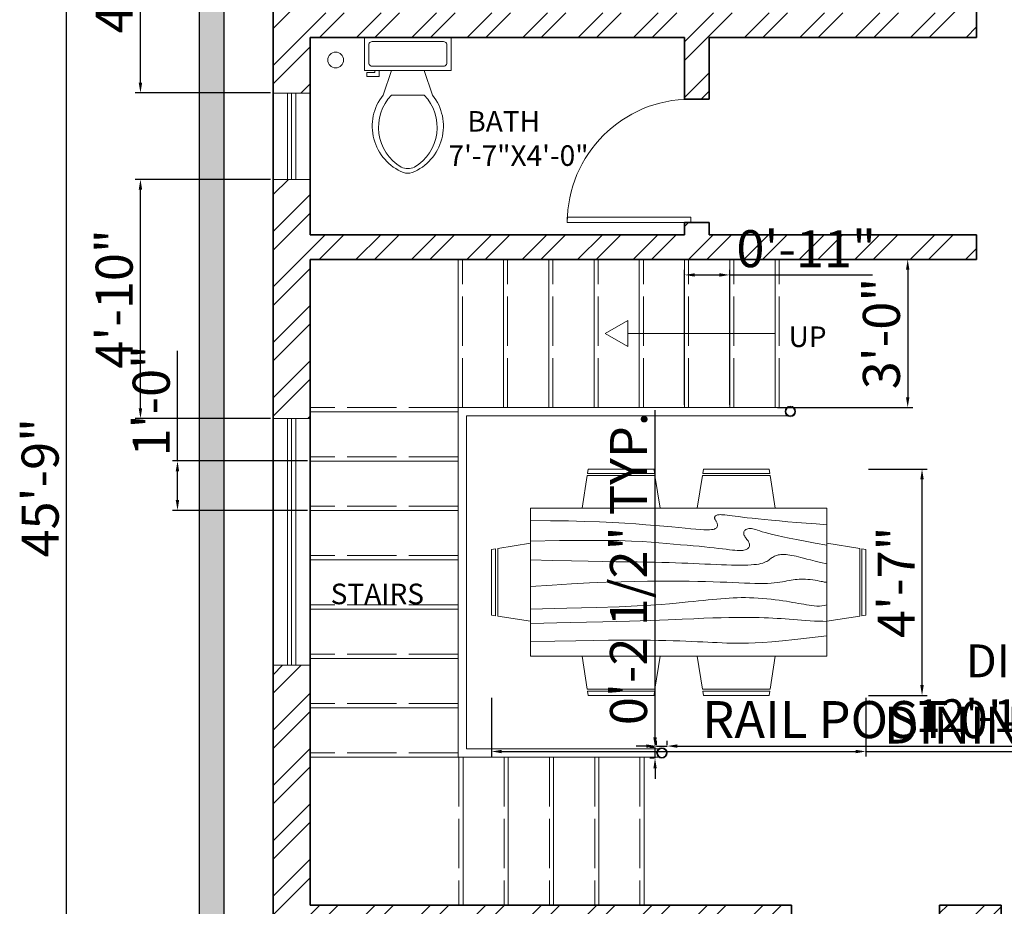
# Model space of a CAD drawing. Units: inches. Extents: x 418 to 1041, y 2094 to 2761.
# Tile 2 of 5: x 484 to 723, y 2308 to 2523. Entities that reach past the tile are written whole.
import ezdxf

# ---------------------------------------------------------------- set-up
doc = ezdxf.new("R2010")
doc.units = ezdxf.units.IN
doc.linetypes.add('ACAD_ISO02W100', pattern=[15, 12, -3])
for name, color, linetype, lineweight in [('A-ANNO-DIMS', 2, 'Continuous', 18), ('A-ANNO-SYMB', 7, 'Continuous', 18), ('A-ANNO-TEXT', 7, 'Continuous', 18), ('A-AREA-IDEN', 7, 'Continuous', 18), ('A-DOOR', 4, 'Continuous', 18), ('A-FLOR-FIXT', 9, 'Continuous', 18), ('A-FLOR-STRS', 7, 'Continuous', 18), ('A-FLOR-STRS-HIDN', 8, 'ACAD_ISO02W100', 13), ('A-FURN', 8, 'Continuous', 18), ('A-GLAZ', 244, 'Continuous', 18), ('A-WALL', 7, 'Continuous', 35), ('A-WALL-PATT', 252, 'Continuous', 13), ('L-WALL', 7, 'Continuous', 25), ('L-WALL-PATT', 252, 'Continuous', 13)]:
    doc.layers.add(name, color=color, linetype=linetype, lineweight=lineweight)
doc.styles.get("Standard").update_dxf_attribs({"font": 'arial.ttf'})
doc.dimstyles.new('ISO-25', dxfattribs={"dimtxt": 9, "dimasz": 2.5, "dimexe": 1.25, "dimexo": 0.625, "dimtad": 1, "dimlunit": 3, "dimtxsty": 'Standard', "dimcen": 2.5, "dimadec": 0, "dimazin": 0, "dimtfac": 1, "dimtmove": 0, "dimatfit": 3, "dimfxl": 1, "dimarcsym": 0})

# ---------------------------------------------------------------- blocks, each defined once
blk = doc.blocks.new('*U6')
for p, q in [((-40, 0), (-40, 6)), ((0, 0), (0, 6))]:
    blk.add_line(p, q)
blk.add_lwpolyline([(0, 0), (0, -40), (-1.75, -40), (-1.75, 0)], close=True)
blk.add_arc((0, 0), 40, 180, 270)
blk = doc.blocks.new('*U10')
for p, q in [((9.5, -6), (9.5, -2)), ((-10, -8.5), (-8, -8.5)), ((-10, -9.5), (-10, -8.5)), ((-7, -9.5), (-10, -9.5)), ((-8, -8.5), (-8, -8)), ((-7, -8), (-7, -9.5)), ((-4, -8), (-6, -14)), ((4, -8), (6, -14)), ((4, -14), (-4, -14))]:
    blk.add_line(p, q)
blk.add_lwpolyline([(10.5, -8), (10.5, 0), (-10.5, 0), (-10.5, -8)], close=True)
for points in [[(-9.5, -2), (-9.5, -6)], [(8.5, -1), (-8.5, -1)], [(-8.5, -7), (8.5, -7)]]:
    blk.add_lwpolyline(points)
for centre, radius, start, end in [((-8.62, -1.88), 0.884, 81.8699, 188.1301), ((8.62, -1.88), 0.884, 351.8699, 98.1301), ((-8.62, -6.12), 0.884, 171.8699, 278.1301), ((8.62, -6.12), 0.884, 261.8699, 8.1301), ((3.52, -21.58), 12.17, 141.4691, 247.9714), ((4.2, -21.82), 11.33, 136.3677, 238.9468), ((-3.52, -21.58), 12.17, 292.0284, 38.5307), ((-4.2, -21.82), 11.33, 301.053, 43.6321), ((0, -27.88), 4, 245.7318, 294.2682), ((0, -29), 4, 254.8605, 285.1395)]:
    blk.add_arc(centre, radius, start, end)
blk = doc.blocks.new('Dining Set - 36 x 72 in.')
for p, q in [((-22, 27.5), (-22.1562, 26.50042)), ((-5.8416, 26.5), (-22.1534, 26.5)), ((-22, 27.5), (-6, 27.5)), ((-5.8437, 26.49966), (-6, 27.5)), ((6, 27.5), (5.8438, 26.50042)), ((22.1584, 26.5), (5.8466, 26.5)), ((6, 27.5), (22, 27.5)), ((22.1563, 26.49966), (22, 27.5)), ((-22.2343, 26.00059), (-23.4847, 17.99762)), ((-22.2304, 26), (-5.7608, 26)), ((-4.5152, 17.99762), (-5.7655, 25.99926)), ((5.7657, 26.00059), (4.5153, 17.99762)), ((5.7696, 26), (22.2392, 26)), ((23.4848, 17.99762), (22.2345, 25.99926)), ((36, 18), (-36, 18)), ((-36, 18), (-36, -18)), ((36, -18), (36, 18)), ((-45.5, 8), (-44.5004, 8.15617)), ((-45.5, 8), (-45.5, -8)), ((-44.5, -8.15843), (-44.5, 8.15338)), ((-44.0006, 8.23428), (-35.9976, 9.48474)), ((-44, 8.23041), (-44, -8.23915)), ((44.0006, 8.23428), (35.9976, 9.48474)), ((44, 8.23041), (44, -8.23915)), ((44.5, -8.15843), (44.5, 8.15338)), ((45.5, 8), (44.5005, 8.15617)), ((45.5, 8), (45.5, -8)), ((-44.4997, -8.15631), (-45.5, -8)), ((-35.9976, -9.48476), (-43.9993, -8.2345)), ((35.9976, -9.48476), (43.9993, -8.2345)), ((44.4997, -8.15631), (45.5, -8)), ((-36, -18), (36, -18)), ((-22.2343, -26.0006), (-23.4847, -17.99762)), ((-4.5152, -17.99762), (-5.7655, -25.99928)), ((5.7657, -26.0006), (4.5153, -17.99762)), ((23.4848, -17.99762), (22.2345, -25.99928)), ((-22.2304, -26), (-5.7608, -26)), ((5.7696, -26), (22.2392, -26)), ((-22, -27.5), (-22.1562, -26.50044)), ((-5.8416, -26.5), (-22.1534, -26.5)), ((-22, -27.5), (-6, -27.5)), ((-5.8437, -26.49967), (-6, -27.5)), ((6, -27.5), (5.8438, -26.50044)), ((22.1584, -26.5), (5.8466, -26.5)), ((6, -27.5), (22, -27.5)), ((22.1563, -26.49967), (22, -27.5))]:
    blk.add_line(p, q)
for points in [[(-36, 15), (-31.1772, 14.97754), (-26.8079, 14.91406), (-22.8538, 14.81543), (-19.276, 14.6875), (-16.0362, 14.53613), (-13.0957, 14.36718), (-10.4159, 14.18652), (-7.9583, 14), (-5.6904, 13.81315), (-3.6035, 13.63021), (-1.6954, 13.45508), (0.0365, 13.29166), (1.5945, 13.14388), (2.9811, 13.01562), (4.1988, 12.9108), (5.25, 12.83333), (6.1393, 12.78613), (6.8802, 12.76823), (7.4883, 12.77767), (7.9792, 12.8125), (8.3685, 12.87077), (8.6719, 12.95052), (8.9049, 13.0498), (9.0833, 13.16666), (9.2205, 13.29899), (9.3216, 13.44401), (9.3895, 13.59879), (9.4271, 13.76041), (9.4373, 13.92594), (9.4232, 14.09245), (9.3875, 14.257), (9.3333, 14.41666), (9.2638, 14.56917), (9.1836, 14.71484), (9.0975, 14.85465), (9.0104, 14.98958), (8.9272, 15.1206), (8.8529, 15.2487), (8.7922, 15.37483), (8.75, 15.5), (8.7305, 15.62467), (8.7344, 15.74739), (8.7617, 15.86621), (8.8125, 15.97916), (8.8867, 16.08431), (8.9844, 16.17968), (9.1055, 16.26334), (9.25, 16.33333), (9.4189, 16.38802), (9.6172, 16.42708), (9.8506, 16.45052), (10.125, 16.45833), (10.4463, 16.45052), (10.8203, 16.42708), (11.2529, 16.38802), (11.75, 16.33333), (12.3184, 16.26318), (12.9694, 16.17838), (13.7151, 16.07991), (14.5677, 15.96875), (15.5395, 15.84586), (16.6426, 15.71224), (17.8893, 15.56884), (19.2917, 15.41666), (20.859, 15.25667), (22.5879, 15.08984), (24.4721, 14.91715), (26.5052, 14.73958), (28.6809, 14.5581), (30.9929, 14.3737), (33.4347, 14.18733), (36, 14)], [(-36, 10), (-28.9766, 10.14274), (-23.1725, 10.20442), (-18.4241, 10.19775), (-14.5677, 10.13541), (-11.4399, 10.03011), (-8.877, 9.89453), (-6.7154, 9.74137), (-4.7917, 9.58333), (-2.9698, 9.43082), (-1.2246, 9.28515), (0.4415, 9.14534), (2.026, 9.01041), (3.5266, 8.87939), (4.9408, 8.7513), (6.266, 8.62516), (7.5, 8.5), (8.6411, 8.37549), (9.6914, 8.2539), (10.6538, 8.13818), (11.5312, 8.03125), (12.3267, 7.93603), (13.043, 7.85547), (13.6831, 7.79248), (14.25, 7.75), (14.7471, 7.7303), (15.1797, 7.73307), (15.5537, 7.75732), (15.875, 7.80208), (16.1494, 7.86637), (16.3828, 7.94922), (16.5811, 8.04964), (16.75, 8.16666), (16.8944, 8.29915), (17.0143, 8.44531), (17.1089, 8.60319), (17.1771, 8.77083), (17.218, 8.94629), (17.2305, 9.1276), (17.2137, 9.31282), (17.1667, 9.5), (17.0895, 9.6875), (16.987, 9.875), (16.8649, 10.0625), (16.7292, 10.25), (16.5856, 10.4375), (16.4401, 10.625), (16.2985, 10.8125), (16.1667, 11), (16.05, 11.18733), (15.9518, 11.3737), (15.8752, 11.5581), (15.8229, 11.73958), (15.798, 11.91715), (15.8034, 12.08984), (15.842, 12.25667), (15.9167, 12.41666), (16.0295, 12.56836), (16.1784, 12.70833), (16.3605, 12.83268), (16.5729, 12.9375), (16.8127, 13.01888), (17.0768, 13.07291), (17.3625, 13.0957), (17.6667, 13.08333), (17.9894, 13.03312), (18.3418, 12.94726), (18.7382, 12.82918), (19.1927, 12.68229), (19.7195, 12.51001), (20.3327, 12.31575), (21.0465, 12.10294), (21.875, 11.875), (22.8357, 11.63354), (23.959, 11.37304), (25.2786, 11.08618), (26.8282, 10.76562), (28.6414, 10.40405), (30.752, 9.99414), (33.1936, 9.52856), (36, 9)], [(-36, 5.5), (-30.7157, 5.3348), (-26.069, 5.20963), (-21.9946, 5.11767), (-18.4271, 5.05208), (-15.3009, 5.00602), (-12.5508, 4.97265), (-10.1112, 4.94515), (-7.9167, 4.91666), (-5.909, 4.88167), (-4.0586, 4.83984), (-2.3429, 4.79215), (-0.7396, 4.73958), (0.7739, 4.6831), (2.22, 4.6237), (3.6213, 4.56233), (5, 4.5), (6.373, 4.43782), (7.7344, 4.3776), (9.0723, 4.32129), (10.375, 4.27083), (11.6309, 4.22819), (12.8281, 4.19531), (13.9551, 4.17415), (15, 4.16666), (15.954, 4.17448), (16.819, 4.19791), (17.6001, 4.23698), (18.3021, 4.29166), (18.9299, 4.36198), (19.4883, 4.44791), (19.9823, 4.54948), (20.4167, 4.66666), (20.7969, 4.79899), (21.1302, 4.94401), (21.4245, 5.09879), (21.6875, 5.26041), (21.9271, 5.42594), (22.1511, 5.59245), (22.3672, 5.757), (22.5834, 5.91666), (22.8065, 6.06868), (23.0404, 6.21093), (23.2879, 6.34147), (23.5521, 6.45833), (23.8358, 6.55957), (24.142, 6.64323), (24.4735, 6.70735), (24.8334, 6.75), (25.2235, 6.76969), (25.642, 6.76692), (26.0858, 6.74267), (26.5521, 6.69791), (27.0379, 6.63362), (27.5404, 6.55078), (28.0565, 6.45036), (28.5834, 6.33333), (29.1242, 6.19987), (29.7071, 6.04687), (30.3661, 5.87044), (31.1354, 5.66666), (32.0493, 5.43164), (33.142, 5.16146), (34.4475, 4.85221), (36, 4.5)], [(-36, -1), (-30.7915, -0.6591), (-26.0195, -0.38216), (-21.6519, -0.16284), (-17.6563, 0.00521), (-14.0005, 0.12833), (-10.6523, 0.21289), (-7.5796, 0.26522), (-4.75, 0.29166), (-2.134, 0.29793), (0.2878, 0.28711), (2.5317, 0.26163), (4.6146, 0.22396), (6.5529, 0.17651), (8.3633, 0.12174), (10.0623, 0.06209), (11.6667, 0), (13.1899, -0.06201), (14.6341, -0.1211), (15.9982, -0.17432), (17.2813, -0.21875), (18.4823, -0.25147), (19.6003, -0.26953), (20.6343, -0.27002), (21.5834, -0.25), (22.4481, -0.20768), (23.2357, -0.14584), (23.9549, -0.06836), (24.6146, 0.02083), (25.2235, 0.11784), (25.7904, 0.21875), (26.3241, 0.31966), (26.8334, 0.41666), (27.3265, 0.50618), (27.8099, 0.58593), (28.2894, 0.65397), (28.7709, 0.70833), (29.2601, 0.74707), (29.763, 0.76823), (30.2855, 0.76985), (30.8334, 0.75), (31.4088, 0.70784), (31.9994, 0.64713), (32.589, 0.57275), (33.1615, 0.48958), (33.7008, 0.4025), (34.1908, 0.3164), (34.6153, 0.23616), (34.9584, 0.16666), (35.2099, 0.11165), (35.3848, 0.07031), (35.504, 0.04069), (35.5886, 0.02083), (35.6594, 0.00879), (35.7377, 0.0026), (35.8442, 0.00032), (36, 0)], [(-36, -6.5), (-27.1843, -6.31267), (-20.084, -6.1263), (-14.469, -5.9419), (-10.1094, -5.76042), (-6.7752, -5.58285), (-4.2363, -5.41016), (-2.2629, -5.24333), (-0.625, -5.08334), (0.8708, -4.93099), (2.2715, -4.78646), (3.5872, -4.64974), (4.8281, -4.52084), (6.0046, -4.39974), (7.127, -4.28646), (8.2053, -4.18099), (9.25, -4.08334), (10.2705, -3.99382), (11.2734, -3.91407), (12.2647, -3.84603), (13.25, -3.79167), (14.2354, -3.75293), (15.2266, -3.73177), (16.2295, -3.73015), (17.25, -3.75), (18.2912, -3.79248), (19.3451, -3.85547), (20.4009, -3.93604), (21.4479, -4.03125), (22.4754, -4.13819), (23.4727, -4.25391), (24.4289, -4.37549), (25.3334, -4.5), (26.1785, -4.62492), (26.9694, -4.74935), (27.7145, -4.87281), (28.4219, -4.99479), (29.1, -5.11483), (29.7572, -5.23242), (30.4016, -5.34709), (31.0417, -5.45834), (31.6837, -5.56437), (32.3262, -5.65821), (32.9658, -5.73153), (33.599, -5.77604), (34.2224, -5.78345), (34.8327, -5.74545), (35.4264, -5.65373), (36, -5.5)], [(-36, -10), (-26.4022, -9.81299), (-18.4675, -9.62891), (-11.9839, -9.45069), (-6.7396, -9.28125), (-2.5226, -9.12354), (0.8789, -8.98047), (3.6769, -8.85498), (6.0833, -8.75), (8.2767, -8.66765), (10.3021, -8.60677), (12.1712, -8.56543), (13.8958, -8.54167), (15.4876, -8.53353), (16.9583, -8.53907), (18.3197, -8.55632), (19.5834, -8.58334), (20.7616, -8.61841), (21.8685, -8.66081), (22.9188, -8.71004), (23.9271, -8.76563), (24.9081, -8.82707), (25.8763, -8.89388), (26.8465, -8.96558), (27.8334, -9.04167), (28.8474, -9.12118), (29.8828, -9.20117), (30.93, -9.27824), (31.9792, -9.34896), (33.0205, -9.40991), (34.0443, -9.45768), (35.0407, -9.48885), (36, -9.5)], [(-36, -14.5), (-30.0881, -14.33513), (-25.0332, -14.21224), (-20.7312, -14.12647), (-17.0781, -14.07292), (-13.97, -14.04671), (-11.3027, -14.04297), (-8.9724, -14.05681), (-6.875, -14.08334), (-4.9224, -14.11833), (-3.0905, -14.16016), (-1.3709, -14.20785), (0.2448, -14.26042), (1.7647, -14.3169), (3.1973, -14.3763), (4.5507, -14.43767), (5.8333, -14.5), (7.0554, -14.5621), (8.235, -14.62175), (9.3922, -14.67652), (10.5469, -14.72396), (11.7192, -14.76164), (12.929, -14.78711), (14.1965, -14.79794), (15.5417, -14.79167), (16.9933, -14.76424), (18.6152, -14.70508), (20.4804, -14.60197), (22.6615, -14.44271), (25.2312, -14.21509), (28.2624, -13.9069), (31.8277, -13.50594), (36, -13)]]:
    blk.add_lwpolyline(points)
blk = doc.blocks.new('WIN-60IN')
for p, q in [((0, 5.5), (60, 5.5)), ((0, 4.5), (60, 4.5)), ((0, 3.5), (60, 3.5))]:
    blk.add_line(p, q)
blk.add_lwpolyline([(0, 9), (60, 9), (60, 0), (0, 0)], close=True)
blk = doc.blocks.new('WIN-21IN')
for p, q in [((0, 5.5), (21, 5.5)), ((0, 4.5), (21, 4.5)), ((0, 3.5), (21, 3.5))]:
    blk.add_line(p, q)
blk.add_lwpolyline([(0, 9), (21, 9), (21, 0), (0, 0)], close=True)
blk = doc.blocks.new('STAIR-RAIL-END-POST')
for radius in [1.28, 1.08]:
    blk.add_circle((1.28, 1.28), radius)
blk = doc.blocks.new('*D33')
at = {"layer": 'A-ANNO-DIMS', "color": 0, "lineweight": -2, "transparency": 16777216}
for p, q in [((638.78, 2346.93), (638.78, 2347.94)), ((641.34, 2346.93), (641.34, 2347.94)), ((636.28, 2346.69), (633.78, 2346.69)), ((638.78, 2346.69), (641.34, 2346.69)), ((643.84, 2346.69), (792.12, 2346.69))]:
    blk.add_line(p, q, dxfattribs=at)
at = {"layer": 'A-ANNO-DIMS', "color": 0, "transparency": 16777216}
for points in [[(636.28, 2347.11), (636.28, 2346.28), (638.78, 2346.69)], [(643.84, 2347.11), (643.84, 2346.28), (641.34, 2346.69)]]:
    blk.add_solid(points, dxfattribs=at)
at = {"layer": 'Defpoints', "color": 0, "transparency": 16777216}
for p in [(638.78, 2346.31), (641.34, 2346.69), (641.34, 2346.31)]:
    blk.add_point(p, dxfattribs=at)
at = {"layer": 'A-ANNO-DIMS', "color": 0, "transparency": 16777216, "insert": (719.23, 2351.97), "char_height": 9, "attachment_point": 5}
blk.add_mtext('RAIL POST 0\'-2 1/2" TYP.', dxfattribs=at)
blk = doc.blocks.new('*D34')
at = {"layer": 'A-ANNO-DIMS', "color": 0, "lineweight": -2, "transparency": 16777216}
for p, q in [((638.39, 2348.81), (638.39, 2428.39)), ((638.15, 2346.31), (637.14, 2346.31)), ((638.39, 2343.75), (638.39, 2346.31)), ((638.15, 2343.75), (637.14, 2343.75)), ((638.39, 2341.25), (638.39, 2338.75))]:
    blk.add_line(p, q, dxfattribs=at)
at = {"layer": 'A-ANNO-DIMS', "color": 0, "transparency": 16777216}
for points in [[(637.98, 2348.81), (638.81, 2348.81), (638.39, 2346.31)], [(637.98, 2341.25), (638.81, 2341.25), (638.39, 2343.75)]]:
    blk.add_solid(points, dxfattribs=at)
at = {"layer": 'Defpoints', "color": 0, "transparency": 16777216}
for p in [(638.39, 2346.31), (638.78, 2346.31), (638.78, 2343.75)]:
    blk.add_point(p, dxfattribs=at)
at = {"layer": 'A-ANNO-DIMS', "color": 0, "transparency": 16777216, "insert": (633.11, 2389.85), "char_height": 9, "attachment_point": 5, "rotation": 90}
blk.add_mtext('0\'-2 1/2" TYP.', dxfattribs=at)
blk = doc.blocks.new('*D35')
at = {"layer": 'A-ANNO-DIMS', "color": 0, "lineweight": -2, "transparency": 16777216}
for p, q in [((598.64, 2358.4), (598.64, 2344.13)), ((689.64, 2358.4), (689.64, 2344.13)), ((601.14, 2345.38), (687.14, 2345.38)), ((689.64, 2345.38), (792.31, 2345.38))]:
    blk.add_line(p, q, dxfattribs=at)
at = {"layer": 'A-ANNO-DIMS', "color": 0, "transparency": 16777216}
for points in [[(601.14, 2345.79), (601.14, 2344.96), (598.64, 2345.38)], [(687.14, 2345.79), (687.14, 2344.96), (689.64, 2345.38)]]:
    blk.add_solid(points, dxfattribs=at)
at = {"layer": 'Defpoints', "color": 0, "transparency": 16777216}
for p in [(598.64, 2359.03), (689.64, 2359.03), (689.64, 2345.38)]:
    blk.add_point(p, dxfattribs=at)
at = {"layer": 'A-ANNO-DIMS', "color": 0, "transparency": 16777216, "insert": (742.22, 2350.65), "char_height": 9, "attachment_point": 5}
blk.add_mtext('DINING SET 7\'-7"', dxfattribs=at)
blk = doc.blocks.new('*D36')
at = {"layer": 'A-ANNO-DIMS', "color": 0, "lineweight": -2, "transparency": 16777216}
for p, q in [((690.26, 2414.03), (704.54, 2414.03)), ((703.29, 2361.53), (703.29, 2411.53)), ((690.26, 2359.03), (704.54, 2359.03))]:
    blk.add_line(p, q, dxfattribs=at)
at = {"layer": 'A-ANNO-DIMS', "color": 0, "transparency": 16777216}
for points in [[(702.87, 2411.53), (703.71, 2411.53), (703.29, 2414.03)], [(702.87, 2361.53), (703.71, 2361.53), (703.29, 2359.03)]]:
    blk.add_solid(points, dxfattribs=at)
at = {"layer": 'Defpoints', "color": 0, "transparency": 16777216}
for p in [(689.64, 2414.03), (703.29, 2414.03), (689.64, 2359.03)]:
    blk.add_point(p, dxfattribs=at)
at = {"layer": 'A-ANNO-DIMS', "color": 0, "transparency": 16777216, "insert": (698.16, 2386.53), "char_height": 9, "attachment_point": 5, "rotation": 90}
blk.add_mtext('4\'-7"', dxfattribs=at)
blk = doc.blocks.new('*D45')
at = {"layer": 'A-ANNO-DIMS', "color": 0, "lineweight": -2, "transparency": 16777216}
for p, q in [((544.93, 2561.61), (512.06, 2561.61)), ((513.31, 2508.03), (513.31, 2559.11)), ((544.93, 2505.53), (512.06, 2505.53))]:
    blk.add_line(p, q, dxfattribs=at)
at = {"layer": 'A-ANNO-DIMS', "color": 0, "transparency": 16777216}
for points in [[(512.89, 2559.11), (513.72, 2559.11), (513.31, 2561.61)], [(512.89, 2508.03), (513.72, 2508.03), (513.31, 2505.53)]]:
    blk.add_solid(points, dxfattribs=at)
at = {"layer": 'Defpoints', "color": 0, "transparency": 16777216}
for p in [(513.31, 2561.61), (545.56, 2561.61), (545.56, 2505.53)]:
    blk.add_point(p, dxfattribs=at)
at = {"layer": 'A-ANNO-DIMS', "color": 0, "transparency": 16777216, "insert": (508.09, 2533.57), "char_height": 9, "attachment_point": 5, "rotation": 90}
blk.add_mtext('4\'-8"', dxfattribs=at)
blk = doc.blocks.new('*D46')
at = {"layer": 'A-ANNO-DIMS', "color": 0, "lineweight": -2, "transparency": 16777216}
for p, q in [((544.93, 2484.53), (512.06, 2484.53)), ((513.31, 2428.85), (513.31, 2482.03)), ((544.93, 2426.35), (512.06, 2426.35))]:
    blk.add_line(p, q, dxfattribs=at)
at = {"layer": 'A-ANNO-DIMS', "color": 0, "transparency": 16777216}
for points in [[(512.89, 2482.03), (513.72, 2482.03), (513.31, 2484.53)], [(512.89, 2428.85), (513.72, 2428.85), (513.31, 2426.35)]]:
    blk.add_solid(points, dxfattribs=at)
at = {"layer": 'Defpoints', "color": 0, "transparency": 16777216}
for p in [(513.31, 2484.53), (545.56, 2484.53), (545.56, 2426.35)]:
    blk.add_point(p, dxfattribs=at)
at = {"layer": 'A-ANNO-DIMS', "color": 0, "transparency": 16777216, "insert": (508.09, 2455.44), "char_height": 9, "attachment_point": 5, "rotation": 90}
blk.add_mtext('4\'-10"', dxfattribs=at)
blk = doc.blocks.new('*D61')
at = {"layer": 'A-ANNO-DIMS', "color": 0, "lineweight": -2, "transparency": 16777216}
for p, q in [((526.93, 2684.03), (494.06, 2684.03)), ((495.31, 2137.53), (495.31, 2681.53)), ((526.93, 2135.03), (494.06, 2135.03))]:
    blk.add_line(p, q, dxfattribs=at)
at = {"layer": 'A-ANNO-DIMS', "color": 0, "transparency": 16777216}
for points in [[(494.89, 2681.53), (495.72, 2681.53), (495.31, 2684.03)], [(494.89, 2137.53), (495.72, 2137.53), (495.31, 2135.03)]]:
    blk.add_solid(points, dxfattribs=at)
at = {"layer": 'Defpoints', "color": 0, "transparency": 16777216}
for p in [(495.31, 2684.03), (527.56, 2684.03), (527.56, 2135.03)]:
    blk.add_point(p, dxfattribs=at)
at = {"layer": 'A-ANNO-DIMS', "color": 0, "transparency": 16777216, "insert": (490.09, 2409.53), "char_height": 9, "attachment_point": 5, "rotation": 90}
blk.add_mtext('45\'-9"', dxfattribs=at)
blk = doc.blocks.new('*D62')
at = {"layer": 'A-ANNO-DIMS', "color": 0, "lineweight": -2, "transparency": 16777216}
for p, q in [((668.18, 2465.03), (701.06, 2465.03)), ((699.81, 2462.53), (699.81, 2431.53)), ((668.18, 2429.03), (701.06, 2429.03))]:
    blk.add_line(p, q, dxfattribs=at)
at = {"layer": 'A-ANNO-DIMS', "color": 0, "transparency": 16777216}
for points in [[(699.39, 2462.53), (700.22, 2462.53), (699.81, 2465.03)], [(699.39, 2431.53), (700.22, 2431.53), (699.81, 2429.03)]]:
    blk.add_solid(points, dxfattribs=at)
at = {"layer": 'Defpoints', "color": 0, "transparency": 16777216}
for p in [(667.56, 2465.03), (667.56, 2429.03), (699.81, 2429.03)]:
    blk.add_point(p, dxfattribs=at)
at = {"layer": 'A-ANNO-DIMS', "color": 0, "transparency": 16777216, "insert": (694.58, 2447.03), "char_height": 9, "attachment_point": 5, "rotation": 90}
blk.add_mtext('3\'-0"', dxfattribs=at)
blk = doc.blocks.new('*D63')
at = {"layer": 'A-ANNO-DIMS', "color": 0, "lineweight": -2, "transparency": 16777216}
for p, q in [((645.56, 2429.65), (645.56, 2462.53)), ((648.06, 2461.28), (654.06, 2461.28)), ((656.56, 2429.65), (656.56, 2462.53)), ((656.56, 2461.28), (691.22, 2461.28))]:
    blk.add_line(p, q, dxfattribs=at)
at = {"layer": 'A-ANNO-DIMS', "color": 0, "transparency": 16777216}
for points in [[(648.06, 2461.69), (648.06, 2460.86), (645.56, 2461.28)], [(654.06, 2461.69), (654.06, 2460.86), (656.56, 2461.28)]]:
    blk.add_solid(points, dxfattribs=at)
at = {"layer": 'Defpoints', "color": 0, "transparency": 16777216}
for p in [(656.56, 2461.28), (645.56, 2429.03), (656.56, 2429.03)]:
    blk.add_point(p, dxfattribs=at)
at = {"layer": 'A-ANNO-DIMS', "color": 0, "transparency": 16777216, "insert": (675.14, 2466.5), "char_height": 9, "attachment_point": 5}
blk.add_mtext('0\'-11"', dxfattribs=at)
blk = doc.blocks.new('*D64')
at = {"layer": 'A-ANNO-DIMS', "color": 0, "lineweight": -2, "transparency": 16777216}
for p, q in [((522.31, 2416.03), (522.31, 2442.85)), ((553.93, 2416.03), (521.06, 2416.03)), ((522.31, 2406.53), (522.31, 2413.53)), ((553.93, 2404.03), (521.06, 2404.03))]:
    blk.add_line(p, q, dxfattribs=at)
at = {"layer": 'A-ANNO-DIMS', "color": 0, "transparency": 16777216}
for points in [[(521.89, 2413.53), (522.72, 2413.53), (522.31, 2416.03)], [(521.89, 2406.53), (522.72, 2406.53), (522.31, 2404.03)]]:
    blk.add_solid(points, dxfattribs=at)
at = {"layer": 'Defpoints', "color": 0, "transparency": 16777216}
for p in [(522.31, 2416.03), (554.56, 2416.03), (554.56, 2404.03)]:
    blk.add_point(p, dxfattribs=at)
at = {"layer": 'A-ANNO-DIMS', "color": 0, "transparency": 16777216, "insert": (517.09, 2430.69), "char_height": 9, "attachment_point": 5, "rotation": 90}
blk.add_mtext('1\'-0"', dxfattribs=at)

msp = doc.modelspace()

# ---------------------------------------------------------------- hatches: boundary and pattern name
at = {"layer": 'A-WALL-PATT'}
h = msp.add_hatch(dxfattribs=at)
h.set_pattern_fill('ANSI32', color=256)
h.paths.add_polyline_path([(671.558, 2308.025), (554.558, 2308.025), (554.558, 2366.352), (545.558, 2366.352), (545.558, 2168.025), (555.667, 2168.025), (555.667, 2177.025), (554.558, 2177.025), (554.558, 2302.025), (671.558, 2302.025)])
h.paths.add_polyline_path([(719.558, 2299.025), (722.558, 2299.025), (722.558, 2306.225), (722.558, 2308.025), (707.558, 2308.025), (707.558, 2302.025), (710.558, 2302.025), (710.558, 2177.025), (665.344, 2177.025), (665.344, 2168.025), (719.558, 2168.025)])
h.paths.add_polyline_path([(605.344, 2177.025), (576.667, 2177.025), (576.667, 2168.025), (605.344, 2168.025)], flags=17)
h.paths.add_polyline_path([(795.654, 2308.025), (770.558, 2308.025), (770.558, 2299.025), (795.654, 2299.025)])
h.paths.add_polyline_path([(971.558, 2333.525), (962.558, 2333.525), (962.558, 2308.025), (890.558, 2308.025), (890.558, 2311.025), (886.058, 2311.025), (884.558, 2311.025), (884.558, 2308.025), (855.654, 2308.025), (855.654, 2299.025), (962.558, 2299.025), (962.558, 2269.763), (971.558, 2269.763)])
h.paths.add_polyline_path([(971.558, 2209.763), (962.558, 2209.763), (962.558, 2168.025), (971.558, 2168.025)])
h.paths.add_polyline_path([(971.558, 2422.525), (962.558, 2422.525), (962.558, 2386.025), (845.558, 2386.025), (845.558, 2380.025), (884.558, 2380.025), (884.558, 2341.025), (890.558, 2341.025), (890.558, 2380.025), (962.558, 2380.025), (962.558, 2354.525), (971.558, 2354.525)])
h.paths.add_polyline_path([(716.558, 2471.025), (651.558, 2471.025), (651.558, 2474.025), (647.058, 2474.025), (645.558, 2474.025), (645.558, 2471.025), (554.558, 2471.025), (554.558, 2484.525), (545.558, 2484.525), (545.558, 2426.352), (554.558, 2426.352), (554.558, 2465.025), (716.558, 2465.025)])
h.paths.add_polyline_path([(554.558, 2561.611), (545.558, 2561.611), (545.558, 2505.525), (554.558, 2505.525), (554.558, 2519.025), (645.558, 2519.025), (645.558, 2504.025), (651.558, 2504.025), (651.558, 2519.025), (716.558, 2519.025), (716.558, 2528.025), (710.558, 2528.025), (710.558, 2525.025), (554.558, 2525.025)])
h.paths.add_polyline_path([(971.558, 2561.025), (962.558, 2561.025), (962.558, 2525.025), (806.558, 2525.025), (806.558, 2528.025), (800.558, 2528.025), (800.558, 2380.025), (809.558, 2380.025), (809.558, 2386.025), (806.558, 2386.025), (806.558, 2519.025), (962.558, 2519.025), (962.558, 2482.525), (971.558, 2482.525)])
h.paths.add_polyline_path([(854.558, 2666.025), (769.058, 2666.025), (769.058, 2657.025), (800.558, 2657.025), (800.558, 2589.025), (797.558, 2589.025), (797.558, 2583.025), (800.558, 2583.025), (800.558, 2564.025), (806.558, 2564.025), (806.558, 2657.025), (854.558, 2657.025)])
h.paths.add_polyline_path([(971.558, 2666.025), (914.558, 2666.025), (914.558, 2657.025), (962.558, 2657.025), (962.558, 2621.025), (971.558, 2621.025)])
h.paths.add_polyline_path([(748.058, 2666.025), (662.558, 2666.025), (662.558, 2657.025), (710.558, 2657.025), (710.558, 2564.025), (716.558, 2564.025), (716.558, 2583.025), (767.558, 2583.025), (767.558, 2589.025), (716.558, 2589.025), (716.558, 2657.025), (748.058, 2657.025)])
h.paths.add_polyline_path([(602.558, 2666.025), (545.558, 2666.025), (545.558, 2621.611), (554.558, 2621.611), (554.558, 2657.025), (602.558, 2657.025)])
at = {"layer": 'L-WALL-PATT'}
h = msp.add_hatch(color=256, dxfattribs=at)
h.dxf.hatch_style = 1
h.paths.add_polyline_path([(533.558, 2678.025), (983.558, 2678.025), (983.558, 2141.025), (902.558, 2141.025), (902.558, 2168.025), (893.558, 2168.025), (893.558, 2135.025), (926.558, 2135.025), (989.558, 2135.025), (989.558, 2684.025), (527.558, 2684.025), (527.558, 2135.025), (723.29, 2135.025), (732.29, 2135.025), (732.29, 2168.025), (723.29, 2168.025), (723.29, 2141.025), (533.558, 2141.025)])

# ---------------------------------------------------------------- linework, layer by layer
at = {"layer": 'A-ANNO-SYMB'}
msp.add_line((667.558, 2447.025), (631.761, 2447.025), dxfattribs=at)
msp.add_lwpolyline([(626.248, 2447.025), (631.761, 2443.842), (631.761, 2450.208)], close=True, dxfattribs=at)
at = {"layer": 'A-FLOR-FIXT'}
msp.add_circle((560.751, 2513.562), 1.921, dxfattribs=at)
at = {"layer": 'A-FLOR-STRS'}
for p, q in [((590.558, 2429.025), (590.558, 2465.025)), ((601.558, 2429.025), (601.558, 2465.025)), ((612.558, 2429.025), (612.558, 2465.025)), ((623.558, 2429.025), (623.558, 2465.025)), ((634.558, 2429.025), (634.558, 2465.025)), ((645.558, 2429.025), (645.558, 2465.025)), ((656.558, 2429.025), (656.558, 2465.025)), ((667.558, 2429.025), (667.558, 2465.025)), ((590.558, 2428.025), (554.558, 2428.025)), ((590.558, 2429.025), (670.405, 2429.025)), ((590.558, 2429.025), (590.558, 2344.025)), ((592.558, 2427.025), (670.553, 2427.025)), ((592.558, 2427.025), (592.558, 2346.025)), ((590.558, 2416.025), (554.558, 2416.025)), ((590.558, 2404.025), (554.558, 2404.025)), ((590.558, 2392.025), (554.558, 2392.025)), ((590.558, 2380.025), (554.558, 2380.025)), ((590.558, 2368.025), (554.558, 2368.025)), ((590.558, 2356.025), (554.558, 2356.025)), ((592.558, 2346.025), (639.254, 2346.025)), ((590.558, 2344.025), (554.558, 2344.025)), ((590.558, 2344.025), (639.262, 2344.025)), ((591.726, 2344.025), (591.726, 2308.025)), ((602.726, 2344.025), (602.726, 2308.025)), ((613.726, 2344.025), (613.726, 2308.025)), ((624.726, 2344.025), (624.726, 2308.025)), ((635.726, 2344.025), (635.726, 2308.025))]:
    msp.add_line(p, q, dxfattribs=at)
at = {"layer": 'A-FLOR-STRS-HIDN'}
for p, q in [((591.558, 2429.025), (591.558, 2465.025)), ((602.558, 2429.025), (602.558, 2465.025)), ((613.558, 2429.025), (613.558, 2465.025)), ((624.558, 2429.025), (624.558, 2465.025)), ((635.558, 2429.025), (635.558, 2465.025)), ((646.558, 2429.025), (646.558, 2465.025)), ((657.558, 2429.025), (657.558, 2465.025)), ((668.558, 2429.025), (668.558, 2465.025)), ((590.558, 2429.025), (554.558, 2429.025)), ((590.558, 2417.025), (554.558, 2417.025)), ((590.558, 2405.025), (554.558, 2405.025)), ((590.558, 2393.025), (554.558, 2393.025)), ((590.558, 2381.025), (554.558, 2381.025)), ((590.558, 2369.025), (554.558, 2369.025)), ((590.558, 2357.025), (554.558, 2357.025)), ((590.558, 2345.025), (554.558, 2345.025)), ((590.726, 2344.025), (590.726, 2308.025)), ((601.726, 2344.025), (601.726, 2308.025)), ((612.726, 2344.025), (612.726, 2308.025)), ((623.726, 2344.025), (623.726, 2308.025)), ((634.726, 2344.025), (634.726, 2308.025))]:
    msp.add_line(p, q, dxfattribs=at)
at = {"layer": 'A-WALL'}
for p, q in [((545.558, 2666.025), (545.558, 2168.025)), ((716.558, 2528.025), (716.558, 2519.025)), ((554.558, 2519.025), (645.558, 2519.025)), ((554.558, 2519.025), (554.558, 2471.025)), ((645.558, 2519.025), (645.558, 2504.025)), ((651.558, 2519.025), (651.558, 2504.025)), ((651.558, 2519.025), (716.558, 2519.025)), ((645.558, 2504.025), (651.558, 2504.025)), ((645.558, 2474.025), (651.558, 2474.025)), ((645.558, 2474.025), (645.558, 2471.025)), ((651.558, 2474.025), (651.558, 2471.025)), ((554.558, 2471.025), (645.558, 2471.025)), ((651.558, 2471.025), (716.558, 2471.025)), ((716.558, 2471.025), (716.558, 2465.025)), ((554.558, 2465.025), (716.558, 2465.025)), ((554.558, 2465.025), (554.558, 2308.025)), ((554.558, 2308.025), (671.558, 2308.025)), ((671.558, 2302.025), (671.558, 2308.025)), ((707.558, 2302.025), (707.558, 2308.025)), ((707.558, 2308.025), (722.558, 2308.025)), ((722.558, 2299.025), (722.558, 2308.025))]:
    msp.add_line(p, q, dxfattribs=at)
at = {"layer": 'L-WALL'}
for p, q in [((527.558, 2684.025), (527.558, 2135.025)), ((533.558, 2678.025), (533.558, 2141.025))]:
    msp.add_line(p, q, dxfattribs=at)

# ---------------------------------------------------------------- block references
at = {"layer": 'A-DOOR', "xscale": 0.75, "yscale": 0.75, "zscale": 0.75, "rotation": 270}
msp.add_blockref('*U6', (647.058, 2474.025), dxfattribs=at)
at = {"layer": 'A-FLOR-FIXT'}
msp.add_blockref('*U10', (578.3, 2519.025), dxfattribs=at)
at = {"layer": 'A-FLOR-STRS'}
for p in [(669.992, 2426.804), (638.777, 2343.749)]:
    msp.add_blockref('STAIR-RAIL-END-POST', p, dxfattribs=at)
at = {"layer": 'A-FURN'}
msp.add_blockref('Dining Set - 36 x 72 in.', (644.139, 2386.525), dxfattribs=at)
at = {"layer": 'A-GLAZ'}
for name, p, rotation in [('WIN-21IN', (545.558, 2505.525), 270.0000000000025), ('WIN-60IN', (545.558, 2426.352), 270.0000000000008)]:
    msp.add_blockref(name, p, dxfattribs=dict(at, rotation=rotation))

# ---------------------------------------------------------------- texts
at = {"layer": 'A-ANNO-TEXT', "insert": (670.845, 2448.754), "char_height": 5, "attachment_point": 1}
msp.add_mtext_dynamic_manual_height_columns('UP', width=9.85826, gutter_width=12.5, heights=[0], dxfattribs=at)
at = {"layer": 'A-AREA-IDEN', "attachment_point": 1}
for s, width, insert, char_height in [('   BATH\\P7\'-7"X4\'-0"', 32.17073, (588.185, 2501.138), 5), ('STAIRS', 25.77056, (559.541, 2386.196), 5), ('     DINING\\P12\'-11"X17\'-1"', 69.88693, (701.72, 2371.422), 8)]:
    msp.add_mtext_dynamic_manual_height_columns(s, width=width, gutter_width=12.5, heights=[0], dxfattribs=dict(at, insert=insert, char_height=char_height))

# ---------------------------------------------------------------- dimensions: what is measured, and where the dimension line sits
at = {"layer": 'A-ANNO-DIMS'}
for base, p1, p2, angle, picture, middle in [((495.308, 2684.025), (527.558, 2135.025), (527.558, 2684.025), 90, '*D61', (490.088, 2409.525)), ((513.308, 2561.611), (545.558, 2505.525), (545.558, 2561.611), 90, '*D45', (508.088, 2533.568)), ((513.308, 2484.525), (545.558, 2426.352), (545.558, 2484.525), 90, '*D46', (508.088, 2455.439)), ((699.808, 2429.025), (667.558, 2465.025), (667.558, 2429.025), 270, '*D62', (694.585, 2447.025)), ((522.308, 2416.025), (554.558, 2404.025), (554.558, 2416.025), 90, '*D64', (517.088, 2430.689)), ((703.289, 2414.025), (689.639, 2359.025), (689.639, 2414.025), 90, '*D36', (698.164, 2386.525))]:
    dim = msp.add_linear_dim(base=base, p1=p1, p2=p2, angle=angle, dimstyle='ISO-25', override={"dimdec": 1, "dimlfac": 1, "dimrnd": 0, "dimzin": 1, "dimdsep": 46, "dimlunit": 4, "dimfrac": 2}, dxfattribs=at)
    dim.commit()
    dim.dimension.update_dxf_attribs({"geometry": picture, "text_midpoint": middle})
dim = msp.add_linear_dim(base=(656.558, 2461.275), p1=(645.558, 2429.025), p2=(656.558, 2429.025), dimstyle='ISO-25', override={"dimdec": 1, "dimlfac": 1, "dimrnd": 0, "dimzin": 1, "dimdsep": 46, "dimlunit": 4, "dimfrac": 2}, dxfattribs=at)
dim.commit()
dim.dimension.update_dxf_attribs({"geometry": '*D63', "text_midpoint": (675.141, 2466.496)})
dim = msp.add_linear_dim(base=(638.393, 2346.309), p1=(638.777, 2343.749), p2=(638.777, 2346.309), angle=90, text='<> TYP.', dimstyle='ISO-25', override={"dimdec": 1, "dimlfac": 1, "dimrnd": 0, "dimzin": 1, "dimdsep": 46, "dimlunit": 4, "dimfrac": 2}, dxfattribs=at)
dim.commit()
dim.dimension.update_dxf_attribs({"geometry": '*D34', "text_midpoint": (633.115, 2389.849)})
for base, p1, p2, text, picture, middle in [((641.337, 2346.693), (638.777, 2346.309), (641.337, 2346.309), 'RAIL POST <> TYP.', '*D33', (719.229, 2351.974)), ((689.639, 2345.375), (598.639, 2359.025), (689.639, 2359.025), 'DINING SET <>', '*D35', (742.225, 2350.654))]:
    dim = msp.add_linear_dim(base=base, p1=p1, p2=p2, text=text, dimstyle='ISO-25', override={"dimdec": 1, "dimlfac": 1, "dimrnd": 0, "dimzin": 1, "dimdsep": 46, "dimlunit": 4, "dimfrac": 2}, dxfattribs=at)
    dim.commit()
    dim.dimension.update_dxf_attribs({"geometry": picture, "text_midpoint": middle})

doc.saveas('drawing.dxf')
